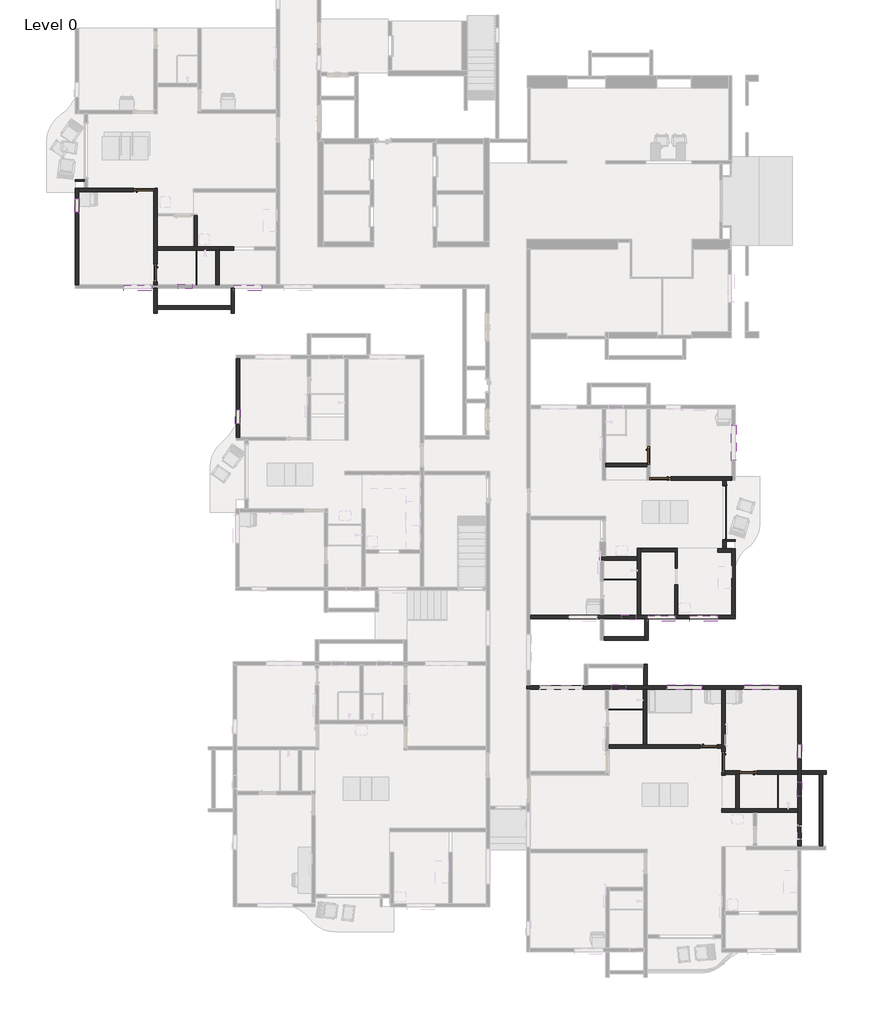
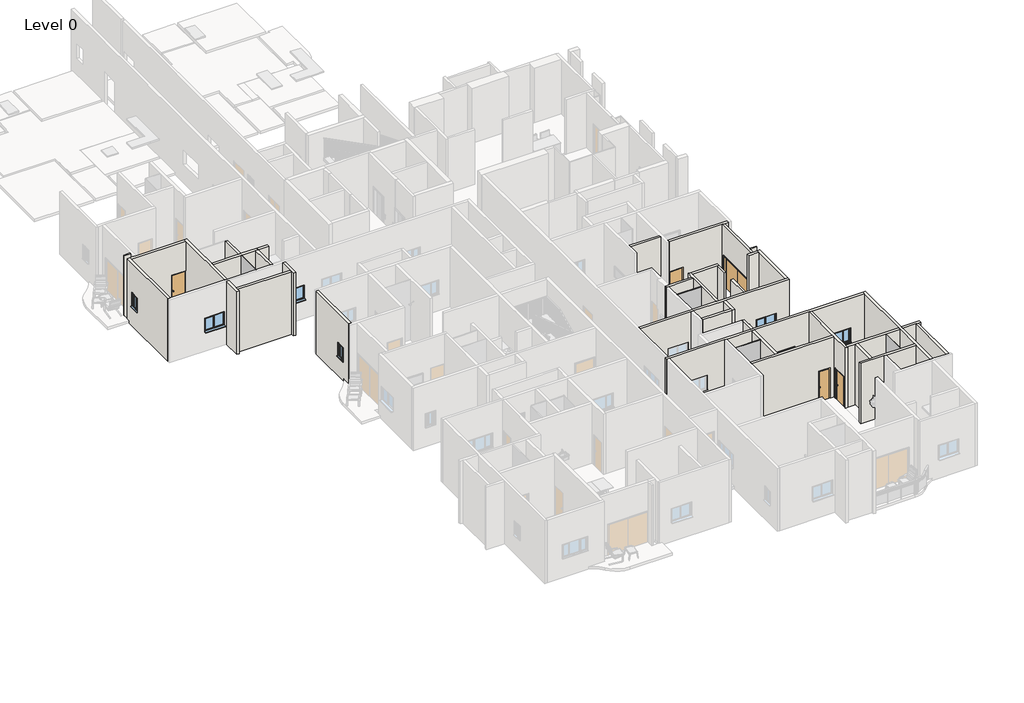
# One storey, part 3 of 14: 35 walls, 14 windows, 8 doors, 4 plates.
# Revit data of these elements (continued)
# Element 1 (IfcDoor, "Doors_Concept_IntDbl : 8'")
#   Phase Created = New Construction
#   Materials on its faces: "Glass", "Glass, Clear Glazing"
# Elements 2, 3, 4 (IfcDoor, "Doors_ExtSgl_Flush : D2")
#   Phase Created = New Construction
#   Materials on its faces: "Door - Handle", "Door - Frame/Mullion", "Door - Panel"
# Elements 5, 6, 7, 8 (IfcDoor, "Doors_ExtSgl_Flush : D3")
#   Phase Created = New Construction
#   Materials on its faces: "Door - Handle", "Door - Frame/Mullion", "Door - Panel"
# Elements 9, 10, 11, 12 (IfcPlate, "System Panel : Glazed")
#   Phase Created = New Construction
#   Materials on its faces: "Glass"
# Elements 13, 14, 15, 16, 17, 18, 19, 20, 21, 22, 23, 24, 25, 26, 27, 28, 29, 30, 31, 32, 33, 34, 35, 36, 37, 38, 39, 40, 41, 42, 43 (IfcWall, "W1")
#   Top Offset = 0 mm
#   Base Offset = 0 mm
#   wall height = 4000 mm
#   Phase Created = New Construction
#   Base Constraint = Level 0
#   Top Constraint = Level 1
#   Materials on its faces: "Brick, Common"
# Elements 44, 45, 46 (IfcWall, "W4")
#   Top Offset = 0 mm
#   Base Offset = 0 mm
#   wall height = 4000 mm
#   Phase Created = New Construction
#   Base Constraint = Level 0
#   Top Constraint = Level 1
#   Materials on its faces: "Brick, Common"
# Element 47 (IfcWall, "W6")
#   Top Offset = 0 mm
#   Base Offset = 0 mm
#   wall height = 4000 mm
#   Phase Created = New Construction
#   Base Constraint = Level 0
#   Top Constraint = Level 1
#   Materials on its faces: "Brick, Common"
# Element 48 (IfcWindow, "Windows_Concept_Plain_Dbl : 4'")
#   Mark = "25"
#   Phase Created = New Construction
#   Materials on its faces: "Window Frame", "Glass"
# Element 49 (IfcWindow, "Windows_Concept_Plain_Dbl : 4'")
#   Mark = "26"
#   Phase Created = New Construction
#   Materials on its faces: "Window Frame", "Glass"
# Element 50 (IfcWindow, "Windows_Concept_Plain_Dbl : 4'")
#   Mark = "54"
#   Phase Created = New Construction
#   Materials on its faces: "Window Frame", "Glass"
# Element 51 (IfcWindow, "Windows_Concept_Plain_Dbl : 4'")
#   Mark = "55"
#   Phase Created = New Construction
#   Materials on its faces: "Window Frame", "Glass"
# Element 52 (IfcWindow, "Windows_Sgl_Plain : 2'")
#   Mark = "21"
#   Phase Created = New Construction
#   Materials on its faces: "Window Frame", "Glass"
# Element 53 (IfcWindow, "Windows_Sgl_Plain : 2'")
#   Mark = "22"
#   Phase Created = New Construction
#   Materials on its faces: "Window Frame", "Glass"
# Element 54 (IfcWindow, "Windows_Sgl_Plain : 2'")
#   Mark = "29"
#   Phase Created = New Construction
#   Materials on its faces: "Window Frame", "Glass"
# Element 55 (IfcWindow, "Windows_Sgl_Plain : 2'")
#   Mark = "57"
#   Phase Created = New Construction
#   Materials on its faces: "Window Frame", "Glass"
# Element 56 (IfcWindow, "Windows_Tpl_Variable_Casement : 2'")
#   Mark = "18"
#   Phase Created = New Construction
#   Materials on its faces: "Window Frame", "Glass"
# Element 57 (IfcWindow, "Windows_Tpl_Variable_Casement : 2'")
#   Mark = "56"
#   Phase Created = New Construction
#   Materials on its faces: "Window Frame", "Glass"
# Element 58 (IfcWindow, "Windows_Tpl_Variable_Casement : 2'")
#   Mark = "63"
#   Phase Created = New Construction
#   Materials on its faces: "Window Frame", "Glass"
# Element 59 (IfcWindow, "Windows_Tpl_Variable_Casement : 5'")
#   Mark = "16"
#   Phase Created = New Construction
#   Materials on its faces: "Window Frame", "Glass"
# Element 60 (IfcWindow, "Windows_Tpl_Variable_Casement : 5'")
#   Mark = "17"
#   Phase Created = New Construction
#   Materials on its faces: "Window Frame", "Glass"
# Element 61 (IfcWindow, "Windows_Tpl_Variable_Casement : 5'")
#   Mark = "27"
#   Phase Created = New Construction
#   Materials on its faces: "Window Frame", "Glass"
# Materials
#   "Glass": class "Glass", colour RGB 0 128 192, transparency 0.9, Description = "Soda Lime Glass", Cost = 0
#   "Glass, Clear Glazing": class "Glass", colour RGB 0 128 192, transparency 0.75, Description = "Clear glazing", Cost = 0
#   "Door - Panel": class "Wood", colour RGB 210 159 95, transparency 0, Keynote = "L20", Cost = 0
#   "Door - Frame/Mullion": class "Wood", colour RGB 212 179 113, transparency 0, Keynote = "L20", Cost = 0
#   "Door - Handle": colour RGB 0 0 0, transparency 0, Keynote = "P21", Cost = 0
#   "Brick, Common": class "Masonry", colour RGB 170 100 105, transparency 0, Description = "Common brick", Cost = 0
#   "Window Frame": colour RGB 249 249 249, transparency 0, Keynote = "L10", Cost = 0
